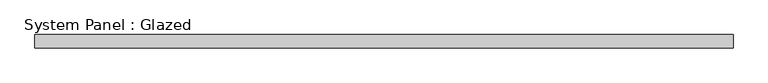
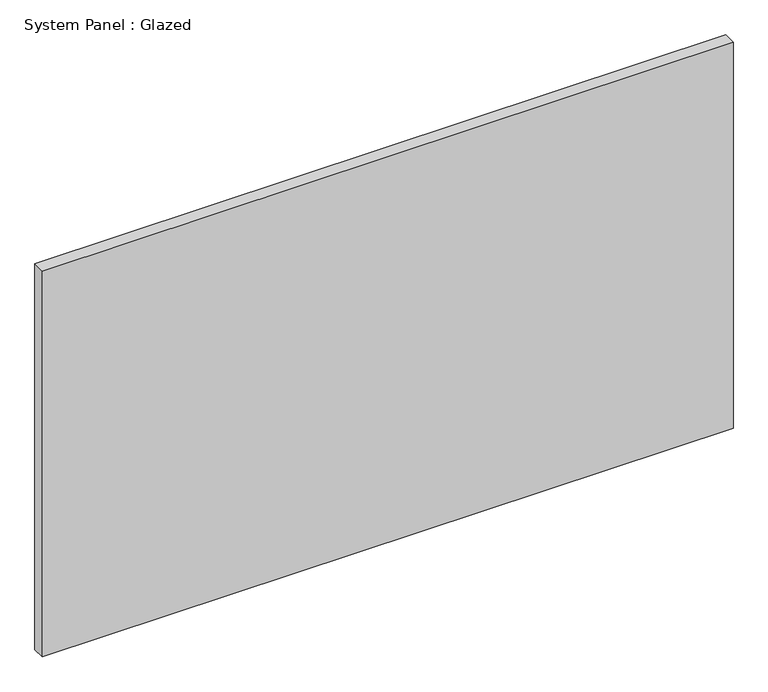
"""IFC4 building model written with IfcOpenShell, lengths in millimetres: plate geometry, System Panel : Glazed."""

from ifc_helpers import new_model, si_unit, origin, origin_with_axes, place, context, project, spatial, polyline, outline, extrude, source, transform, mapped, element, save


def system_panel_glazed_baedfebd(model_context):
    return source(origin(), model_context, "Body", "SweptSolid", [
        extrude(outline(polyline([(676.275, 19.05), (-676.275, 19.05), (-676.275, 44.45), (676.275, 44.45), (676.275, 19.05)])), origin_with_axes(), (0.0, 0.0, 1.0), 798.9054943),
    ])


if __name__ == "__main__":
    model = new_model("IFC4")
    model_context = context("Model", 3, world=origin())
    ifc_project = project(units=[si_unit("LENGTHUNIT", "METRE", prefix="MILLI")], contexts=[model_context])
    site = spatial("IfcSite", under=ifc_project)
    building = spatial("IfcBuilding", under=site)
    placement = place(None, origin())
    system_panel_glazed_shape = system_panel_glazed_baedfebd(model_context)
    element("IfcPlate", 1, ObjectType="System Panel : Glazed", at=placement, inside=building, context=model_context, shape_type="MappedRepresentation", body=[
        mapped(system_panel_glazed_shape, transform((0.0, 0.0, 0.0), x_axis=(1.0, 0.0, 0.0), y_axis=(0.0, 1.0, 0.0), z_axis=(0.0, 0.0, 1.0))),
    ])
    save(model, "model.ifc")

# Revit data of these elements
# Type "System Panel : Glazed"
#   Construction Type Id = "GSP4R"
#   Analytic Construction = "1/8 in Pilkington single glazing"
#   Visual Light Transmittance = 0.9
#   Solar Heat Gain Coefficient = 0.86
#   Heat Transfer Coefficient (U) = 1.18115 BTU/(h·ft²·°F)
#   Define Thermal Properties by = 1
# Element 1 (IfcPlate, "System Panel : Glazed")
#   Materials on its faces: "Glass"
# Materials
#   "Glass": class "Glass", colour RGB 0 128 192, transparency 0.75, Description = "Soda Lime Glass", Cost = 0
